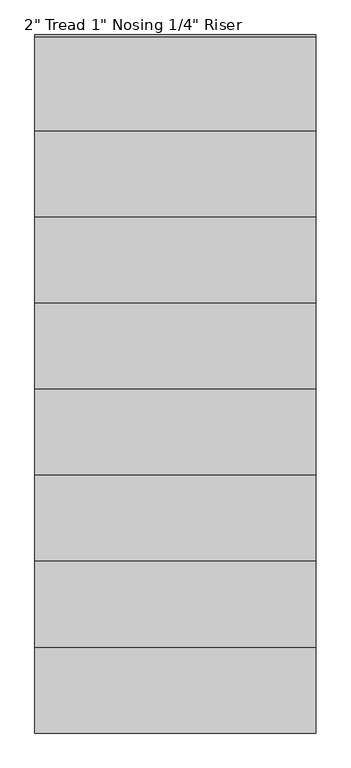
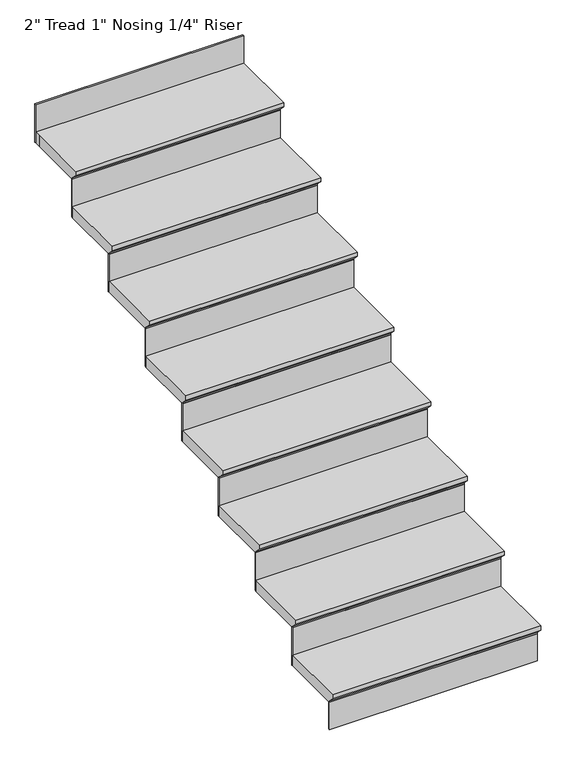
"""IFC4 building model written with IfcOpenShell, lengths in millimetres: stair flight geometry."""

from ifc_helpers import new_model, si_unit, origin, place, context, project, spatial, faceted_brep, source, transform, mapped, element, save


def stair_flight_485682bc(model_context):
    return source(origin(), model_context, "Body", "Brep", [
        faceted_brep([(-11728.968339, 6177.243496, 7169.15), (-11728.968339, 6177.243496, 7188.2), (-12643.368339, 6177.243496, 7188.2), (-12643.368339, 6177.243496, 7169.15), (-11728.968339, 6202.643496, 7143.75), (-12643.368339, 6202.643496, 7143.75), (-11728.968339, 6482.043496, 7188.2), (-12643.368339, 6482.043496, 7188.2), (-12643.368339, 6202.643496, 7137.4), (-12643.368339, 6482.043496, 7137.4), (-11728.968339, 6482.043496, 7137.4), (-11728.968339, 6202.643496, 7137.4)], [[[0, 1, 2, 3]], [[4, 0, 3, 5]], [[2, 1, 6, 7]], [[8, 9, 10, 11]], [[2, 7, 9, 8, 5, 3]], [[8, 11, 4, 5]], [[6, 1, 0, 4, 11, 10]], [[7, 6, 10, 9]]]),
        faceted_brep([(-11728.968339, 6202.643496, 7137.4), (-11728.968339, 6202.643496, 7010.4), (-11728.968339, 6208.993496, 7010.4), (-11728.968339, 6208.993496, 7137.4), (-12643.368339, 6202.643496, 7137.4), (-12643.368339, 6208.993496, 7137.4), (-12643.368339, 6208.993496, 7010.4), (-12643.368339, 6202.643496, 7010.4)], [[[0, 1, 2, 3]], [[4, 5, 6, 7]], [[1, 0, 4, 7]], [[2, 1, 7, 6]], [[3, 2, 6, 5]], [[0, 3, 5, 4]]]),
        faceted_brep([(-11728.968339, 6482.043496, 7315.2), (-11728.968339, 6482.043496, 7137.4), (-11728.968339, 6488.393496, 7137.4), (-11728.968339, 6488.393496, 7315.2), (-12643.368339, 6482.043496, 7315.2), (-12643.368339, 6488.393496, 7315.2), (-12643.368339, 6488.393496, 7137.4), (-12643.368339, 6482.043496, 7137.4)], [[[0, 1, 2, 3]], [[4, 5, 6, 7]], [[1, 0, 4, 7]], [[2, 1, 7, 6]], [[3, 2, 6, 5]], [[0, 3, 5, 4]]]),
        faceted_brep([(-12643.368339, 6456.643496, 7366.0), (-11728.968339, 6456.643496, 7366.0), (-11728.968339, 6761.443496, 7366.0), (-12643.368339, 6761.443496, 7366.0), (-12643.368339, 6482.043496, 7315.2), (-12643.368339, 6761.443496, 7315.2), (-11728.968339, 6761.443496, 7315.2), (-11728.968339, 6482.043496, 7315.2), (-12643.368339, 6482.043496, 7321.55), (-12643.368339, 6456.643496, 7346.95), (-11728.968339, 6482.043496, 7321.55), (-11728.968339, 6456.643496, 7346.95)], [[[0, 1, 2, 3]], [[4, 5, 6, 7]], [[0, 3, 5, 4, 8, 9]], [[4, 7, 10, 8]], [[2, 1, 11, 10, 7, 6]], [[3, 2, 6, 5]], [[11, 1, 0, 9]], [[10, 11, 9, 8]]]),
        faceted_brep([(-11728.968339, 6761.443496, 7493.0), (-11728.968339, 6761.443496, 7315.2), (-11728.968339, 6767.793496, 7315.2), (-11728.968339, 6767.793496, 7493.0), (-12643.368339, 6761.443496, 7493.0), (-12643.368339, 6767.793496, 7493.0), (-12643.368339, 6767.793496, 7315.2), (-12643.368339, 6761.443496, 7315.2)], [[[0, 1, 2, 3]], [[4, 5, 6, 7]], [[1, 0, 4, 7]], [[2, 1, 7, 6]], [[3, 2, 6, 5]], [[0, 3, 5, 4]]]),
        faceted_brep([(-12643.368339, 6736.043496, 7543.8), (-11728.968339, 6736.043496, 7543.8), (-11728.968339, 7040.843496, 7543.8), (-12643.368339, 7040.843496, 7543.8), (-12643.368339, 6761.443496, 7493.0), (-12643.368339, 7040.843496, 7493.0), (-11728.968339, 7040.843496, 7493.0), (-11728.968339, 6761.443496, 7493.0), (-12643.368339, 6761.443496, 7499.35), (-12643.368339, 6736.043496, 7524.75), (-11728.968339, 6761.443496, 7499.35), (-11728.968339, 6736.043496, 7524.75)], [[[0, 1, 2, 3]], [[4, 5, 6, 7]], [[0, 3, 5, 4, 8, 9]], [[4, 7, 10, 8]], [[2, 1, 11, 10, 7, 6]], [[3, 2, 6, 5]], [[11, 1, 0, 9]], [[10, 11, 9, 8]]]),
        faceted_brep([(-11728.968339, 7040.843496, 7670.8), (-11728.968339, 7040.843496, 7493.0), (-11728.968339, 7047.193496, 7493.0), (-11728.968339, 7047.193496, 7670.8), (-12643.368339, 7040.843496, 7670.8), (-12643.368339, 7047.193496, 7670.8), (-12643.368339, 7047.193496, 7493.0), (-12643.368339, 7040.843496, 7493.0)], [[[0, 1, 2, 3]], [[4, 5, 6, 7]], [[1, 0, 4, 7]], [[2, 1, 7, 6]], [[3, 2, 6, 5]], [[0, 3, 5, 4]]]),
        faceted_brep([(-12643.368339, 7015.443496, 7721.6), (-11728.968339, 7015.443496, 7721.6), (-11728.968339, 7320.243496, 7721.6), (-12643.368339, 7320.243496, 7721.6), (-12643.368339, 7040.843496, 7670.8), (-12643.368339, 7320.243496, 7670.8), (-11728.968339, 7320.243496, 7670.8), (-11728.968339, 7040.843496, 7670.8), (-12643.368339, 7040.843496, 7677.15), (-12643.368339, 7015.443496, 7702.55), (-11728.968339, 7040.843496, 7677.15), (-11728.968339, 7015.443496, 7702.55)], [[[0, 1, 2, 3]], [[4, 5, 6, 7]], [[0, 3, 5, 4, 8, 9]], [[4, 7, 10, 8]], [[2, 1, 11, 10, 7, 6]], [[3, 2, 6, 5]], [[11, 1, 0, 9]], [[10, 11, 9, 8]]]),
        faceted_brep([(-11728.968339, 7320.243496, 7848.6), (-11728.968339, 7320.243496, 7670.8), (-11728.968339, 7326.593496, 7670.8), (-11728.968339, 7326.593496, 7848.6), (-12643.368339, 7320.243496, 7848.6), (-12643.368339, 7326.593496, 7848.6), (-12643.368339, 7326.593496, 7670.8), (-12643.368339, 7320.243496, 7670.8)], [[[0, 1, 2, 3]], [[4, 5, 6, 7]], [[1, 0, 4, 7]], [[2, 1, 7, 6]], [[3, 2, 6, 5]], [[0, 3, 5, 4]]]),
        faceted_brep([(-12643.368339, 7294.843496, 7899.4), (-11728.968339, 7294.843496, 7899.4), (-11728.968339, 7599.643496, 7899.4), (-12643.368339, 7599.643496, 7899.4), (-12643.368339, 7320.243496, 7848.6), (-12643.368339, 7599.643496, 7848.6), (-11728.968339, 7599.643496, 7848.6), (-11728.968339, 7320.243496, 7848.6), (-12643.368339, 7320.243496, 7854.95), (-12643.368339, 7294.843496, 7880.35), (-11728.968339, 7320.243496, 7854.95), (-11728.968339, 7294.843496, 7880.35)], [[[0, 1, 2, 3]], [[4, 5, 6, 7]], [[0, 3, 5, 4, 8, 9]], [[4, 7, 10, 8]], [[2, 1, 11, 10, 7, 6]], [[3, 2, 6, 5]], [[11, 1, 0, 9]], [[10, 11, 9, 8]]]),
        faceted_brep([(-11728.968339, 7599.643496, 8026.4), (-11728.968339, 7599.643496, 7848.6), (-11728.968339, 7605.993496, 7848.6), (-11728.968339, 7605.993496, 8026.4), (-12643.368339, 7599.643496, 8026.4), (-12643.368339, 7605.993496, 8026.4), (-12643.368339, 7605.993496, 7848.6), (-12643.368339, 7599.643496, 7848.6)], [[[0, 1, 2, 3]], [[4, 5, 6, 7]], [[1, 0, 4, 7]], [[2, 1, 7, 6]], [[3, 2, 6, 5]], [[0, 3, 5, 4]]]),
        faceted_brep([(-12643.368339, 7574.243496, 8077.2), (-11728.968339, 7574.243496, 8077.2), (-11728.968339, 7879.043496, 8077.2), (-12643.368339, 7879.043496, 8077.2), (-12643.368339, 7599.643496, 8026.4), (-12643.368339, 7879.043496, 8026.4), (-11728.968339, 7879.043496, 8026.4), (-11728.968339, 7599.643496, 8026.4), (-12643.368339, 7599.643496, 8032.75), (-12643.368339, 7574.243496, 8058.15), (-11728.968339, 7599.643496, 8032.75), (-11728.968339, 7574.243496, 8058.15)], [[[0, 1, 2, 3]], [[4, 5, 6, 7]], [[0, 3, 5, 4, 8, 9]], [[4, 7, 10, 8]], [[2, 1, 11, 10, 7, 6]], [[3, 2, 6, 5]], [[11, 1, 0, 9]], [[10, 11, 9, 8]]]),
        faceted_brep([(-11728.968339, 7879.043496, 8204.2), (-11728.968339, 7879.043496, 8026.4), (-11728.968339, 7885.393496, 8026.4), (-11728.968339, 7885.393496, 8204.2), (-12643.368339, 7879.043496, 8204.2), (-12643.368339, 7885.393496, 8204.2), (-12643.368339, 7885.393496, 8026.4), (-12643.368339, 7879.043496, 8026.4)], [[[0, 1, 2, 3]], [[4, 5, 6, 7]], [[1, 0, 4, 7]], [[2, 1, 7, 6]], [[3, 2, 6, 5]], [[0, 3, 5, 4]]]),
        faceted_brep([(-12643.368339, 7853.643496, 8255.0), (-11728.968339, 7853.643496, 8255.0), (-11728.968339, 8158.443496, 8255.0), (-12643.368339, 8158.443496, 8255.0), (-12643.368339, 7879.043496, 8204.2), (-12643.368339, 8158.443496, 8204.2), (-11728.968339, 8158.443496, 8204.2), (-11728.968339, 7879.043496, 8204.2), (-12643.368339, 7879.043496, 8210.55), (-12643.368339, 7853.643496, 8235.95), (-11728.968339, 7879.043496, 8210.55), (-11728.968339, 7853.643496, 8235.95)], [[[0, 1, 2, 3]], [[4, 5, 6, 7]], [[0, 3, 5, 4, 8, 9]], [[4, 7, 10, 8]], [[2, 1, 11, 10, 7, 6]], [[3, 2, 6, 5]], [[11, 1, 0, 9]], [[10, 11, 9, 8]]]),
        faceted_brep([(-11728.968339, 8437.843496, 8559.8), (-11728.968339, 8437.843496, 8382.0), (-11728.968339, 8444.193496, 8382.0), (-11728.968339, 8444.193496, 8559.8), (-12643.368339, 8437.843496, 8559.8), (-12643.368339, 8444.193496, 8559.8), (-12643.368339, 8444.193496, 8382.0), (-12643.368339, 8437.843496, 8382.0)], [[[0, 1, 2, 3]], [[4, 5, 6, 7]], [[1, 0, 4, 7]], [[2, 1, 7, 6]], [[3, 2, 6, 5]], [[0, 3, 5, 4]]]),
        faceted_brep([(-11728.968339, 8158.443496, 8382.0), (-11728.968339, 8158.443496, 8204.2), (-11728.968339, 8164.793496, 8204.2), (-11728.968339, 8164.793496, 8382.0), (-12643.368339, 8158.443496, 8382.0), (-12643.368339, 8164.793496, 8382.0), (-12643.368339, 8164.793496, 8204.2), (-12643.368339, 8158.443496, 8204.2)], [[[0, 1, 2, 3]], [[4, 5, 6, 7]], [[1, 0, 4, 7]], [[2, 1, 7, 6]], [[3, 2, 6, 5]], [[0, 3, 5, 4]]]),
        faceted_brep([(-12643.368339, 8437.843496, 8432.8), (-12643.368339, 8412.443496, 8432.8), (-12643.368339, 8133.043496, 8432.8), (-11728.968339, 8133.043496, 8432.8), (-11728.968339, 8437.843496, 8432.8), (-12643.368339, 8412.443496, 8382.0), (-12643.368339, 8437.843496, 8382.0), (-11728.968339, 8437.843496, 8382.0), (-11728.968339, 8158.443496, 8382.0), (-12643.368339, 8158.443496, 8382.0), (-12643.368339, 8158.443496, 8388.35), (-12643.368339, 8133.043496, 8413.75), (-11728.968339, 8158.443496, 8388.35), (-11728.968339, 8133.043496, 8413.75)], [[[0, 1, 2, 3, 4]], [[5, 6, 7, 8, 9]], [[1, 0, 6, 5]], [[2, 1, 5, 9, 10, 11]], [[9, 8, 12, 10]], [[4, 3, 13, 12, 8, 7]], [[0, 4, 7, 6]], [[13, 3, 2, 11]], [[12, 13, 11, 10]]]),
    ])


if __name__ == "__main__":
    model = new_model("IFC4")
    model_context = context("Model", 3, world=origin())
    ifc_project = project(units=[si_unit("LENGTHUNIT", "METRE", prefix="MILLI")], contexts=[model_context])
    site = spatial("IfcSite", under=ifc_project)
    building = spatial("IfcBuilding", under=site)
    placement = place(None, origin())
    stair_flight_shape = stair_flight_485682bc(model_context)
    element("IfcStairFlight", 1, ObjectType="2\" Tread 1\" Nosing 1/4\" Riser", at=placement, inside=building, context=model_context, shape_type="MappedRepresentation", body=[
        mapped(stair_flight_shape, transform((0.0, 0.0, 0.0), x_axis=(1.0, 0.0, 0.0), y_axis=(0.0, 1.0, 0.0), z_axis=(0.0, 0.0, 1.0))),
    ])
    save(model, "model.ifc")
